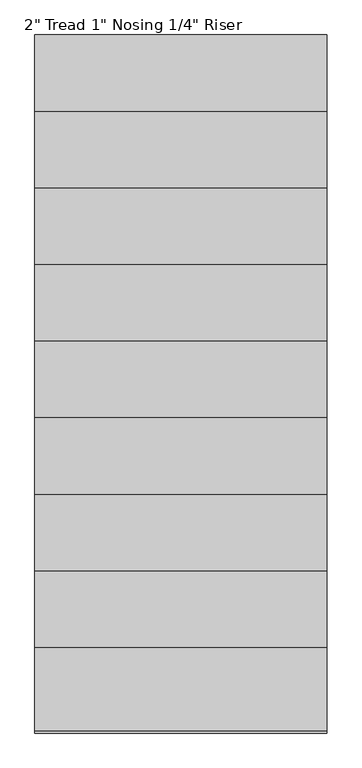
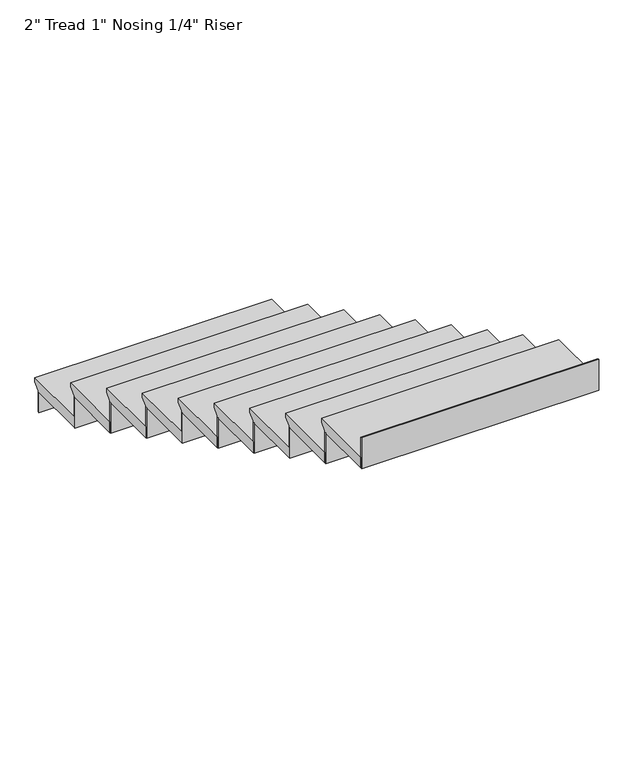
"""IFC4 building model written with IfcOpenShell, lengths in millimetres: stair flight geometry."""

from ifc_helpers import new_model, si_unit, origin, place, context, project, spatial, faceted_brep, source, transform, mapped, element, save


def stair_flight_1f098d2d(model_context):
    return source(origin(), model_context, "Body", "Brep", [
        faceted_brep([(-16114.6847893, 12510.5922903, 126.4227273), (-16114.6847893, 12510.5922903, 145.4727273), (-15047.8847893, 12510.5922903, 145.4727273), (-15047.8847893, 12510.5922903, 126.4227273), (-16114.6847893, 12485.1922903, 101.0227273), (-15047.8847893, 12485.1922903, 101.0227273), (-16114.6847893, 12205.7922903, 145.4727273), (-15047.8847893, 12205.7922903, 145.4727273), (-15047.8847893, 12485.1922903, 94.6727273), (-15047.8847893, 12205.7922903, 94.6727273), (-16114.6847893, 12205.7922903, 94.6727273), (-16114.6847893, 12485.1922903, 94.6727273)], [[[0, 1, 2, 3]], [[4, 0, 3, 5]], [[2, 1, 6, 7]], [[8, 9, 10, 11]], [[2, 7, 9, 8, 5, 3]], [[8, 11, 4, 5]], [[6, 1, 0, 4, 11, 10]], [[7, 6, 10, 9]]]),
        faceted_brep([(-16114.6847893, 12485.1922903, 94.6727273), (-16114.6847893, 12485.1922903, 0.0), (-16114.6847893, 12478.8422903, 0.0), (-16114.6847893, 12478.8422903, 94.6727273), (-15047.8847893, 12485.1922903, 94.6727273), (-15047.8847893, 12478.8422903, 94.6727273), (-15047.8847893, 12478.8422903, 0.0), (-15047.8847893, 12485.1922903, 0.0)], [[[0, 1, 2, 3]], [[4, 5, 6, 7]], [[1, 0, 4, 7]], [[2, 1, 7, 6]], [[3, 2, 6, 5]], [[0, 3, 5, 4]]]),
        faceted_brep([(-16114.6847893, 12205.7922903, 240.1454545), (-16114.6847893, 12205.7922903, 94.6727273), (-16114.6847893, 12199.4422903, 94.6727273), (-16114.6847893, 12199.4422903, 240.1454545), (-15047.8847893, 12205.7922903, 240.1454545), (-15047.8847893, 12199.4422903, 240.1454545), (-15047.8847893, 12199.4422903, 94.6727273), (-15047.8847893, 12205.7922903, 94.6727273)], [[[0, 1, 2, 3]], [[4, 5, 6, 7]], [[1, 0, 4, 7]], [[2, 1, 7, 6]], [[3, 2, 6, 5]], [[0, 3, 5, 4]]]),
        faceted_brep([(-15047.8847893, 12231.1922903, 290.9454545), (-16114.6847893, 12231.1922903, 290.9454545), (-16114.6847893, 11926.3922903, 290.9454545), (-15047.8847893, 11926.3922903, 290.9454545), (-15047.8847893, 12205.7922903, 240.1454545), (-15047.8847893, 11926.3922903, 240.1454545), (-16114.6847893, 11926.3922903, 240.1454545), (-16114.6847893, 12205.7922903, 240.1454545), (-15047.8847893, 12205.7922903, 246.4954545), (-15047.8847893, 12231.1922903, 271.8954545), (-16114.6847893, 12205.7922903, 246.4954545), (-16114.6847893, 12231.1922903, 271.8954545)], [[[0, 1, 2, 3]], [[4, 5, 6, 7]], [[0, 3, 5, 4, 8, 9]], [[4, 7, 10, 8]], [[2, 1, 11, 10, 7, 6]], [[3, 2, 6, 5]], [[11, 1, 0, 9]], [[10, 11, 9, 8]]]),
        faceted_brep([(-16114.6847893, 11926.3922903, 385.6181818), (-16114.6847893, 11926.3922903, 240.1454545), (-16114.6847893, 11920.0422903, 240.1454545), (-16114.6847893, 11920.0422903, 385.6181818), (-15047.8847893, 11926.3922903, 385.6181818), (-15047.8847893, 11920.0422903, 385.6181818), (-15047.8847893, 11920.0422903, 240.1454545), (-15047.8847893, 11926.3922903, 240.1454545)], [[[0, 1, 2, 3]], [[4, 5, 6, 7]], [[1, 0, 4, 7]], [[2, 1, 7, 6]], [[3, 2, 6, 5]], [[0, 3, 5, 4]]]),
        faceted_brep([(-15047.8847893, 11951.7922903, 436.4181818), (-16114.6847893, 11951.7922903, 436.4181818), (-16114.6847893, 11646.9922903, 436.4181818), (-15047.8847893, 11646.9922903, 436.4181818), (-15047.8847893, 11926.3922903, 385.6181818), (-15047.8847893, 11646.9922903, 385.6181818), (-16114.6847893, 11646.9922903, 385.6181818), (-16114.6847893, 11926.3922903, 385.6181818), (-15047.8847893, 11926.3922903, 391.9681818), (-15047.8847893, 11951.7922903, 417.3681818), (-16114.6847893, 11926.3922903, 391.9681818), (-16114.6847893, 11951.7922903, 417.3681818)], [[[0, 1, 2, 3]], [[4, 5, 6, 7]], [[0, 3, 5, 4, 8, 9]], [[4, 7, 10, 8]], [[2, 1, 11, 10, 7, 6]], [[3, 2, 6, 5]], [[11, 1, 0, 9]], [[10, 11, 9, 8]]]),
        faceted_brep([(-16114.6847893, 11646.9922903, 531.0909091), (-16114.6847893, 11646.9922903, 385.6181818), (-16114.6847893, 11640.6422903, 385.6181818), (-16114.6847893, 11640.6422903, 531.0909091), (-15047.8847893, 11646.9922903, 531.0909091), (-15047.8847893, 11640.6422903, 531.0909091), (-15047.8847893, 11640.6422903, 385.6181818), (-15047.8847893, 11646.9922903, 385.6181818)], [[[0, 1, 2, 3]], [[4, 5, 6, 7]], [[1, 0, 4, 7]], [[2, 1, 7, 6]], [[3, 2, 6, 5]], [[0, 3, 5, 4]]]),
        faceted_brep([(-15047.8847893, 11672.3922903, 581.8909091), (-16114.6847893, 11672.3922903, 581.8909091), (-16114.6847893, 11367.5922903, 581.8909091), (-15047.8847893, 11367.5922903, 581.8909091), (-15047.8847893, 11646.9922903, 531.0909091), (-15047.8847893, 11367.5922903, 531.0909091), (-16114.6847893, 11367.5922903, 531.0909091), (-16114.6847893, 11646.9922903, 531.0909091), (-15047.8847893, 11646.9922903, 537.4409091), (-15047.8847893, 11672.3922903, 562.8409091), (-16114.6847893, 11646.9922903, 537.4409091), (-16114.6847893, 11672.3922903, 562.8409091)], [[[0, 1, 2, 3]], [[4, 5, 6, 7]], [[0, 3, 5, 4, 8, 9]], [[4, 7, 10, 8]], [[2, 1, 11, 10, 7, 6]], [[3, 2, 6, 5]], [[11, 1, 0, 9]], [[10, 11, 9, 8]]]),
        faceted_brep([(-16114.6847893, 11367.5922903, 676.5636364), (-16114.6847893, 11367.5922903, 531.0909091), (-16114.6847893, 11361.2422903, 531.0909091), (-16114.6847893, 11361.2422903, 676.5636364), (-15047.8847893, 11367.5922903, 676.5636364), (-15047.8847893, 11361.2422903, 676.5636364), (-15047.8847893, 11361.2422903, 531.0909091), (-15047.8847893, 11367.5922903, 531.0909091)], [[[0, 1, 2, 3]], [[4, 5, 6, 7]], [[1, 0, 4, 7]], [[2, 1, 7, 6]], [[3, 2, 6, 5]], [[0, 3, 5, 4]]]),
        faceted_brep([(-15047.8847893, 11392.9922903, 727.3636364), (-16114.6847893, 11392.9922903, 727.3636364), (-16114.6847893, 11088.1922903, 727.3636364), (-15047.8847893, 11088.1922903, 727.3636364), (-15047.8847893, 11367.5922903, 676.5636364), (-15047.8847893, 11088.1922903, 676.5636364), (-16114.6847893, 11088.1922903, 676.5636364), (-16114.6847893, 11367.5922903, 676.5636364), (-15047.8847893, 11367.5922903, 682.9136364), (-15047.8847893, 11392.9922903, 708.3136364), (-16114.6847893, 11367.5922903, 682.9136364), (-16114.6847893, 11392.9922903, 708.3136364)], [[[0, 1, 2, 3]], [[4, 5, 6, 7]], [[0, 3, 5, 4, 8, 9]], [[4, 7, 10, 8]], [[2, 1, 11, 10, 7, 6]], [[3, 2, 6, 5]], [[11, 1, 0, 9]], [[10, 11, 9, 8]]]),
        faceted_brep([(-16114.6847893, 11088.1922903, 822.0363636), (-16114.6847893, 11088.1922903, 676.5636364), (-16114.6847893, 11081.8422903, 676.5636364), (-16114.6847893, 11081.8422903, 822.0363636), (-15047.8847893, 11088.1922903, 822.0363636), (-15047.8847893, 11081.8422903, 822.0363636), (-15047.8847893, 11081.8422903, 676.5636364), (-15047.8847893, 11088.1922903, 676.5636364)], [[[0, 1, 2, 3]], [[4, 5, 6, 7]], [[1, 0, 4, 7]], [[2, 1, 7, 6]], [[3, 2, 6, 5]], [[0, 3, 5, 4]]]),
        faceted_brep([(-15047.8847893, 11113.5922903, 872.8363636), (-16114.6847893, 11113.5922903, 872.8363636), (-16114.6847893, 10808.7922903, 872.8363636), (-15047.8847893, 10808.7922903, 872.8363636), (-15047.8847893, 11088.1922903, 822.0363636), (-15047.8847893, 10808.7922903, 822.0363636), (-16114.6847893, 10808.7922903, 822.0363636), (-16114.6847893, 11088.1922903, 822.0363636), (-15047.8847893, 11088.1922903, 828.3863636), (-15047.8847893, 11113.5922903, 853.7863636), (-16114.6847893, 11088.1922903, 828.3863636), (-16114.6847893, 11113.5922903, 853.7863636)], [[[0, 1, 2, 3]], [[4, 5, 6, 7]], [[0, 3, 5, 4, 8, 9]], [[4, 7, 10, 8]], [[2, 1, 11, 10, 7, 6]], [[3, 2, 6, 5]], [[11, 1, 0, 9]], [[10, 11, 9, 8]]]),
        faceted_brep([(-16114.6847893, 10808.7922903, 967.5090909), (-16114.6847893, 10808.7922903, 822.0363636), (-16114.6847893, 10802.4422903, 822.0363636), (-16114.6847893, 10802.4422903, 967.5090909), (-15047.8847893, 10808.7922903, 967.5090909), (-15047.8847893, 10802.4422903, 967.5090909), (-15047.8847893, 10802.4422903, 822.0363636), (-15047.8847893, 10808.7922903, 822.0363636)], [[[0, 1, 2, 3]], [[4, 5, 6, 7]], [[1, 0, 4, 7]], [[2, 1, 7, 6]], [[3, 2, 6, 5]], [[0, 3, 5, 4]]]),
        faceted_brep([(-15047.8847893, 10834.1922903, 1018.3090909), (-16114.6847893, 10834.1922903, 1018.3090909), (-16114.6847893, 10529.3922903, 1018.3090909), (-15047.8847893, 10529.3922903, 1018.3090909), (-15047.8847893, 10808.7922903, 967.5090909), (-15047.8847893, 10529.3922903, 967.5090909), (-16114.6847893, 10529.3922903, 967.5090909), (-16114.6847893, 10808.7922903, 967.5090909), (-15047.8847893, 10808.7922903, 973.8590909), (-15047.8847893, 10834.1922903, 999.2590909), (-16114.6847893, 10808.7922903, 973.8590909), (-16114.6847893, 10834.1922903, 999.2590909)], [[[0, 1, 2, 3]], [[4, 5, 6, 7]], [[0, 3, 5, 4, 8, 9]], [[4, 7, 10, 8]], [[2, 1, 11, 10, 7, 6]], [[3, 2, 6, 5]], [[11, 1, 0, 9]], [[10, 11, 9, 8]]]),
        faceted_brep([(-16114.6847893, 10529.3922903, 1112.9818182), (-16114.6847893, 10529.3922903, 967.5090909), (-16114.6847893, 10523.0422903, 967.5090909), (-16114.6847893, 10523.0422903, 1112.9818182), (-15047.8847893, 10529.3922903, 1112.9818182), (-15047.8847893, 10523.0422903, 1112.9818182), (-15047.8847893, 10523.0422903, 967.5090909), (-15047.8847893, 10529.3922903, 967.5090909)], [[[0, 1, 2, 3]], [[4, 5, 6, 7]], [[1, 0, 4, 7]], [[2, 1, 7, 6]], [[3, 2, 6, 5]], [[0, 3, 5, 4]]]),
        faceted_brep([(-15047.8847893, 10554.7922903, 1163.7818182), (-16114.6847893, 10554.7922903, 1163.7818182), (-16114.6847893, 10249.9922903, 1163.7818182), (-15047.8847893, 10249.9922903, 1163.7818182), (-15047.8847893, 10529.3922903, 1112.9818182), (-15047.8847893, 10249.9922903, 1112.9818182), (-16114.6847893, 10249.9922903, 1112.9818182), (-16114.6847893, 10529.3922903, 1112.9818182), (-15047.8847893, 10529.3922903, 1119.3318182), (-15047.8847893, 10554.7922903, 1144.7318182), (-16114.6847893, 10529.3922903, 1119.3318182), (-16114.6847893, 10554.7922903, 1144.7318182)], [[[0, 1, 2, 3]], [[4, 5, 6, 7]], [[0, 3, 5, 4, 8, 9]], [[4, 7, 10, 8]], [[2, 1, 11, 10, 7, 6]], [[3, 2, 6, 5]], [[11, 1, 0, 9]], [[10, 11, 9, 8]]]),
        faceted_brep([(-16114.6847893, 9970.5922903, 1403.9272727), (-16114.6847893, 9970.5922903, 1258.4545455), (-16114.6847893, 9964.2422903, 1258.4545455), (-16114.6847893, 9964.2422903, 1403.9272727), (-15047.8847893, 9970.5922903, 1403.9272727), (-15047.8847893, 9964.2422903, 1403.9272727), (-15047.8847893, 9964.2422903, 1258.4545455), (-15047.8847893, 9970.5922903, 1258.4545455)], [[[0, 1, 2, 3]], [[4, 5, 6, 7]], [[1, 0, 4, 7]], [[2, 1, 7, 6]], [[3, 2, 6, 5]], [[0, 3, 5, 4]]]),
        faceted_brep([(-16114.6847893, 10249.9922903, 1258.4545455), (-16114.6847893, 10249.9922903, 1112.9818182), (-16114.6847893, 10243.6422903, 1112.9818182), (-16114.6847893, 10243.6422903, 1258.4545455), (-15047.8847893, 10249.9922903, 1258.4545455), (-15047.8847893, 10243.6422903, 1258.4545455), (-15047.8847893, 10243.6422903, 1112.9818182), (-15047.8847893, 10249.9922903, 1112.9818182)], [[[0, 1, 2, 3]], [[4, 5, 6, 7]], [[1, 0, 4, 7]], [[2, 1, 7, 6]], [[3, 2, 6, 5]], [[0, 3, 5, 4]]]),
        faceted_brep([(-15047.8847893, 9970.5922903, 1309.2545455), (-15047.8847893, 9995.9922903, 1309.2545455), (-15047.8847893, 10275.3922903, 1309.2545455), (-16114.6847893, 10275.3922903, 1309.2545455), (-16114.6847893, 9970.5922903, 1309.2545455), (-15047.8847893, 9995.9922903, 1258.4545455), (-15047.8847893, 9970.5922903, 1258.4545455), (-16114.6847893, 9970.5922903, 1258.4545455), (-16114.6847893, 10249.9922903, 1258.4545455), (-15047.8847893, 10249.9922903, 1258.4545455), (-15047.8847893, 10249.9922903, 1264.8045455), (-15047.8847893, 10275.3922903, 1290.2045455), (-16114.6847893, 10249.9922903, 1264.8045455), (-16114.6847893, 10275.3922903, 1290.2045455)], [[[0, 1, 2, 3, 4]], [[5, 6, 7, 8, 9]], [[1, 0, 6, 5]], [[2, 1, 5, 9, 10, 11]], [[9, 8, 12, 10]], [[4, 3, 13, 12, 8, 7]], [[0, 4, 7, 6]], [[13, 3, 2, 11]], [[12, 13, 11, 10]]]),
    ])


if __name__ == "__main__":
    model = new_model("IFC4")
    model_context = context("Model", 3, world=origin())
    ifc_project = project(units=[si_unit("LENGTHUNIT", "METRE", prefix="MILLI")], contexts=[model_context])
    site = spatial("IfcSite", under=ifc_project)
    building = spatial("IfcBuilding", under=site)
    placement = place(None, origin())
    stair_flight_shape = stair_flight_1f098d2d(model_context)
    element("IfcStairFlight", 1, ObjectType="2\" Tread 1\" Nosing 1/4\" Riser", at=placement, inside=building, context=model_context, shape_type="MappedRepresentation", body=[
        mapped(stair_flight_shape, transform((0.0, 0.0, 0.0), x_axis=(1.0, 0.0, 0.0), y_axis=(0.0, 1.0, 0.0), z_axis=(0.0, 0.0, 1.0))),
    ])
    save(model, "model.ifc")
